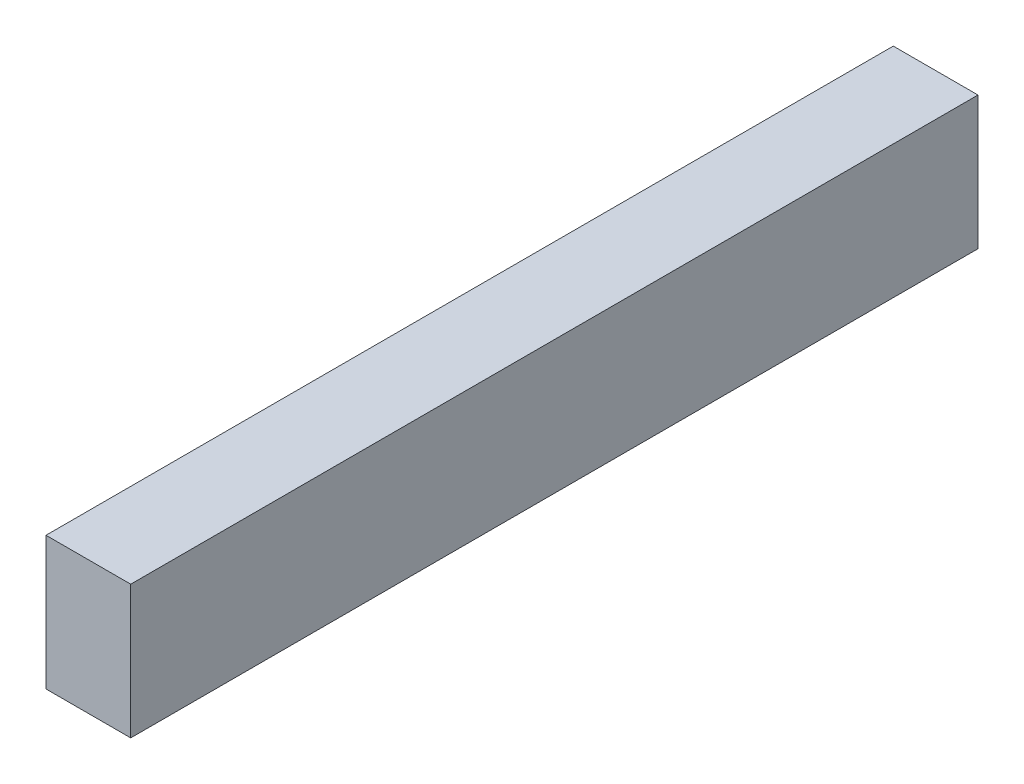
ISO-10303-21;
HEADER;
FILE_DESCRIPTION(('STEP AP214'),'2;1');
FILE_NAME('part.step','',(''),(''),'','','');
FILE_SCHEMA(('AUTOMOTIVE_DESIGN { 1 0 10303 214 1 1 1 1 }'));
ENDSEC;
DATA;
#1=APPLICATION_CONTEXT('core data for automotive mechanical design processes');
#2=APPLICATION_PROTOCOL_DEFINITION('international standard','automotive_design',2000,#1);
#3=PRODUCT_CONTEXT('',#1,'mechanical');
#4=PRODUCT('Part','Part','',(#3));
#5=PRODUCT_RELATED_PRODUCT_CATEGORY('part','',(#4));
#6=PRODUCT_DEFINITION_FORMATION('','',#4);
#7=PRODUCT_DEFINITION_CONTEXT('part definition',#1,'design');
#8=PRODUCT_DEFINITION('design','',#6,#7);
#9=PRODUCT_DEFINITION_SHAPE('','',#8);
#10=(LENGTH_UNIT() NAMED_UNIT(*) SI_UNIT(.MILLI.,.METRE.));
#11=(NAMED_UNIT(*) PLANE_ANGLE_UNIT() SI_UNIT($,.RADIAN.));
#12=(NAMED_UNIT(*) SI_UNIT($,.STERADIAN.) SOLID_ANGLE_UNIT());
#13=UNCERTAINTY_MEASURE_WITH_UNIT(LENGTH_MEASURE(1.E-05),#10,'distance_accuracy_value','');
#14=(GEOMETRIC_REPRESENTATION_CONTEXT(3) GLOBAL_UNCERTAINTY_ASSIGNED_CONTEXT((#13)) GLOBAL_UNIT_ASSIGNED_CONTEXT((#10,
#11,#12)) REPRESENTATION_CONTEXT('',''));
#15=CARTESIAN_POINT('',(0.,0.,0.));
#16=DIRECTION('',(0.,0.,1.));
#17=DIRECTION('',(1.,0.,0.));
#18=AXIS2_PLACEMENT_3D('',#15,#16,#17);
#19=CARTESIAN_POINT('',(6.99999999999999,-11.,70.));
#20=DIRECTION('',(-1.,0.,0.));
#21=DIRECTION('',(0.,0.,1.));
#22=AXIS2_PLACEMENT_3D('',#19,#20,#21);
#23=PLANE('',#22);
#24=DIRECTION('',(0.,1.,0.));
#25=VECTOR('',#24,1.);
#26=CARTESIAN_POINT('',(6.99999999999999,-11.,-70.));
#27=LINE('',#26,#25);
#28=CARTESIAN_POINT('',(6.99999999999999,-11.,-70.));
#29=VERTEX_POINT('',#28);
#30=CARTESIAN_POINT('',(6.99999999999999,11.,-70.));
#31=VERTEX_POINT('',#30);
#32=EDGE_CURVE('E105',#29,#31,#27,.T.);
#33=ORIENTED_EDGE('',*,*,#32,.T.);
#34=DIRECTION('',(0.,0.,-1.));
#35=VECTOR('',#34,1.);
#36=CARTESIAN_POINT('',(6.99999999999999,11.,70.));
#37=LINE('',#36,#35);
#38=CARTESIAN_POINT('',(6.99999999999999,11.,70.));
#39=VERTEX_POINT('',#38);
#40=EDGE_CURVE('E11',#39,#31,#37,.T.);
#41=ORIENTED_EDGE('',*,*,#40,.F.);
#42=DIRECTION('',(0.,1.,0.));
#43=VECTOR('',#42,1.);
#44=CARTESIAN_POINT('',(6.99999999999999,-11.,70.));
#45=LINE('',#44,#43);
#46=CARTESIAN_POINT('',(6.99999999999999,-11.,70.));
#47=VERTEX_POINT('',#46);
#48=EDGE_CURVE('E89',#47,#39,#45,.T.);
#49=ORIENTED_EDGE('',*,*,#48,.F.);
#50=DIRECTION('',(0.,0.,-1.));
#51=VECTOR('',#50,1.);
#52=CARTESIAN_POINT('',(6.99999999999999,-11.,70.));
#53=LINE('',#52,#51);
#54=EDGE_CURVE('E98',#47,#29,#53,.T.);
#55=ORIENTED_EDGE('',*,*,#54,.T.);
#56=EDGE_LOOP('',(#33,#41,#49,#55));
#57=FACE_BOUND('',#56,.T.);
#58=ADVANCED_FACE('F39',(#57),#23,.F.);
#59=CARTESIAN_POINT('',(-7.,11.,70.));
#60=DIRECTION('',(0.,-1.,0.));
#61=DIRECTION('',(0.,0.,-1.));
#62=AXIS2_PLACEMENT_3D('',#59,#60,#61);
#63=PLANE('',#62);
#64=DIRECTION('',(-1.,0.,0.));
#65=VECTOR('',#64,1.);
#66=CARTESIAN_POINT('',(-7.,11.,-70.));
#67=LINE('',#66,#65);
#68=CARTESIAN_POINT('',(-7.,11.,-70.));
#69=VERTEX_POINT('',#68);
#70=EDGE_CURVE('E94',#31,#69,#67,.T.);
#71=ORIENTED_EDGE('',*,*,#70,.T.);
#72=DIRECTION('',(0.,0.,-1.));
#73=VECTOR('',#72,1.);
#74=CARTESIAN_POINT('',(-7.,11.,70.));
#75=LINE('',#74,#73);
#76=CARTESIAN_POINT('',(-7.,11.,70.));
#77=VERTEX_POINT('',#76);
#78=EDGE_CURVE('E50',#77,#69,#75,.T.);
#79=ORIENTED_EDGE('',*,*,#78,.F.);
#80=DIRECTION('',(-1.,0.,0.));
#81=VECTOR('',#80,1.);
#82=CARTESIAN_POINT('',(-7.,11.,70.));
#83=LINE('',#82,#81);
#84=EDGE_CURVE('E83',#39,#77,#83,.T.);
#85=ORIENTED_EDGE('',*,*,#84,.F.);
#86=ORIENTED_EDGE('',*,*,#40,.T.);
#87=EDGE_LOOP('',(#71,#79,#85,#86));
#88=FACE_BOUND('',#87,.T.);
#89=ADVANCED_FACE('F91',(#88),#63,.F.);
#90=CARTESIAN_POINT('',(-7.,-11.,70.));
#91=DIRECTION('',(1.,0.,0.));
#92=DIRECTION('',(0.,0.,-1.));
#93=AXIS2_PLACEMENT_3D('',#90,#91,#92);
#94=PLANE('',#93);
#95=DIRECTION('',(0.,-1.,0.));
#96=VECTOR('',#95,1.);
#97=CARTESIAN_POINT('',(-7.,-11.,-70.));
#98=LINE('',#97,#96);
#99=CARTESIAN_POINT('',(-7.,-11.,-70.));
#100=VERTEX_POINT('',#99);
#101=EDGE_CURVE('E75',#69,#100,#98,.T.);
#102=ORIENTED_EDGE('',*,*,#101,.T.);
#103=DIRECTION('',(0.,0.,-1.));
#104=VECTOR('',#103,1.);
#105=CARTESIAN_POINT('',(-7.,-11.,70.));
#106=LINE('',#105,#104);
#107=CARTESIAN_POINT('',(-7.,-11.,70.));
#108=VERTEX_POINT('',#107);
#109=EDGE_CURVE('E92',#108,#100,#106,.T.);
#110=ORIENTED_EDGE('',*,*,#109,.F.);
#111=DIRECTION('',(0.,-1.,0.));
#112=VECTOR('',#111,1.);
#113=CARTESIAN_POINT('',(-7.,-11.,70.));
#114=LINE('',#113,#112);
#115=EDGE_CURVE('E86',#77,#108,#114,.T.);
#116=ORIENTED_EDGE('',*,*,#115,.F.);
#117=ORIENTED_EDGE('',*,*,#78,.T.);
#118=EDGE_LOOP('',(#102,#110,#116,#117));
#119=FACE_BOUND('',#118,.T.);
#120=ADVANCED_FACE('F96',(#119),#94,.F.);
#121=CARTESIAN_POINT('',(-7.,-11.,70.));
#122=DIRECTION('',(0.,1.,0.));
#123=DIRECTION('',(0.,0.,1.));
#124=AXIS2_PLACEMENT_3D('',#121,#122,#123);
#125=PLANE('',#124);
#126=DIRECTION('',(1.,0.,0.));
#127=VECTOR('',#126,1.);
#128=CARTESIAN_POINT('',(-7.,-11.,-70.));
#129=LINE('',#128,#127);
#130=EDGE_CURVE('E79',#100,#29,#129,.T.);
#131=ORIENTED_EDGE('',*,*,#130,.T.);
#132=ORIENTED_EDGE('',*,*,#54,.F.);
#133=DIRECTION('',(1.,0.,0.));
#134=VECTOR('',#133,1.);
#135=CARTESIAN_POINT('',(-7.,-11.,70.));
#136=LINE('',#135,#134);
#137=EDGE_CURVE('E54',#108,#47,#136,.T.);
#138=ORIENTED_EDGE('',*,*,#137,.F.);
#139=ORIENTED_EDGE('',*,*,#109,.T.);
#140=EDGE_LOOP('',(#131,#132,#138,#139));
#141=FACE_BOUND('',#140,.T.);
#142=ADVANCED_FACE('F108',(#141),#125,.F.);
#143=CARTESIAN_POINT('',(0.,0.,70.));
#144=DIRECTION('',(0.,0.,-1.));
#145=DIRECTION('',(-1.,0.,0.));
#146=AXIS2_PLACEMENT_3D('',#143,#144,#145);
#147=PLANE('',#146);
#148=ORIENTED_EDGE('',*,*,#48,.T.);
#149=ORIENTED_EDGE('',*,*,#84,.T.);
#150=ORIENTED_EDGE('',*,*,#115,.T.);
#151=ORIENTED_EDGE('',*,*,#137,.T.);
#152=EDGE_LOOP('',(#148,#149,#150,#151));
#153=FACE_BOUND('',#152,.T.);
#154=ADVANCED_FACE('F88',(#153),#147,.F.);
#155=CARTESIAN_POINT('',(0.,0.,-70.));
#156=DIRECTION('',(0.,0.,-1.));
#157=DIRECTION('',(-1.,0.,0.));
#158=AXIS2_PLACEMENT_3D('',#155,#156,#157);
#159=PLANE('',#158);
#160=ORIENTED_EDGE('',*,*,#32,.F.);
#161=ORIENTED_EDGE('',*,*,#130,.F.);
#162=ORIENTED_EDGE('',*,*,#101,.F.);
#163=ORIENTED_EDGE('',*,*,#70,.F.);
#164=EDGE_LOOP('',(#160,#161,#162,#163));
#165=FACE_BOUND('',#164,.T.);
#166=ADVANCED_FACE('F115',(#165),#159,.T.);
#167=CLOSED_SHELL('',(#58,#89,#120,#142,#154,#166));
#168=MANIFOLD_SOLID_BREP('B2',#167);
#169=ADVANCED_BREP_SHAPE_REPRESENTATION('',(#18,#168),#14);
#170=SHAPE_DEFINITION_REPRESENTATION(#9,#169);
ENDSEC;
END-ISO-10303-21;
